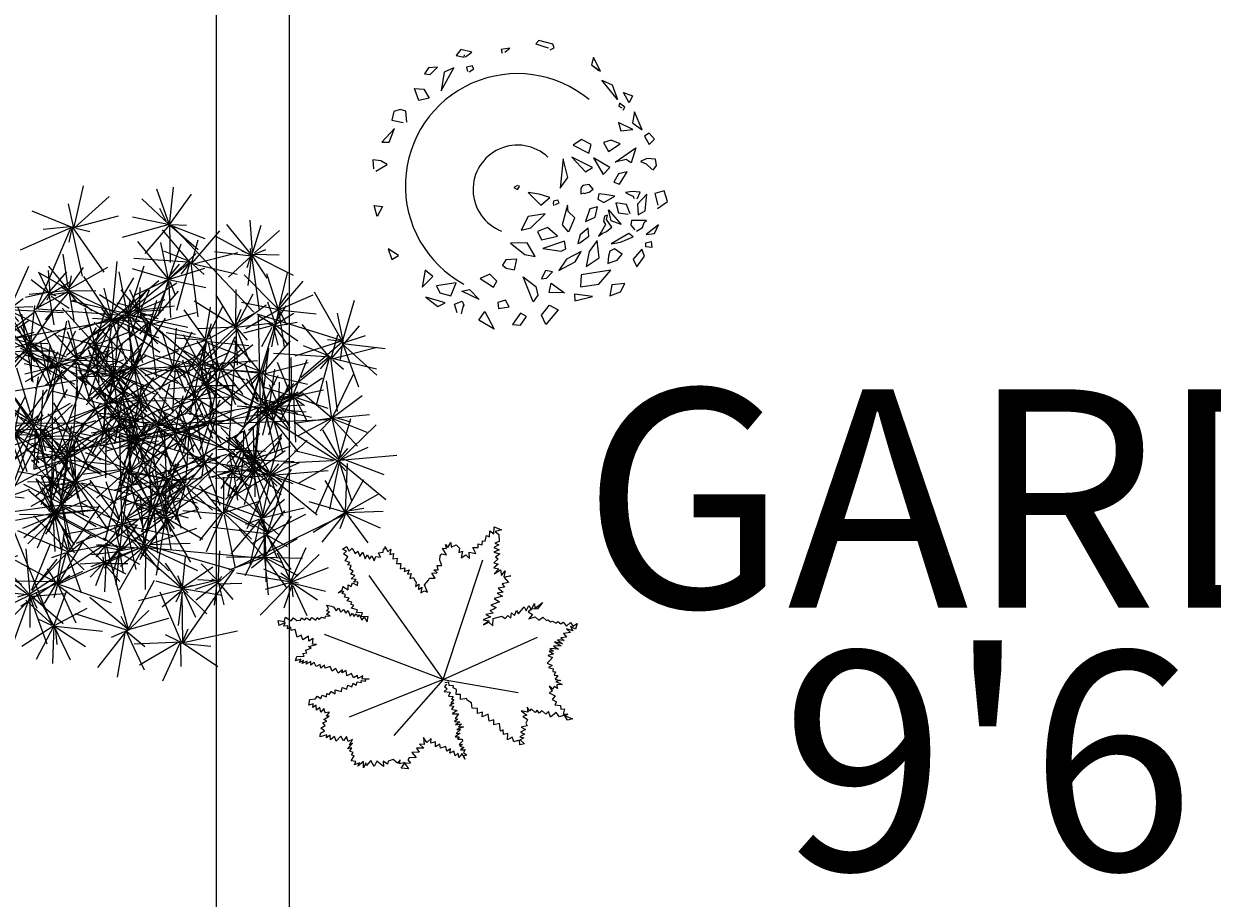
# Model space of a CAD drawing. Units: inches. Extents: x 8049 to 8459, y 820 to 1350.
# Tile 15 of 25: x 8132 to 8165, y 906 to 930. Entities that reach past the tile are written whole.
import ezdxf

# ---------------------------------------------------------------- set-up
doc = ezdxf.new("R2010")
doc.units = ezdxf.units.IN
doc.header["$MEASUREMENT"] = 0
for name, color, linetype, lineweight in [('A-ANNO-DIMS', 2, 'Continuous', 18), ('A-AREA-IDEN', 7, 'Continuous', 25), ('zelen', 69, 'Continuous', 13)]:
    doc.layers.add(name, color=color, linetype=linetype, lineweight=lineweight)
doc.styles.get("Standard").update_dxf_attribs({"font": 'arial.ttf'})
doc.dimstyles.get("Standard").update_dxf_attribs({"dimtxt": 0.18, "dimasz": 0.18, "dimexe": 0.18, "dimexo": 0.0625, "dimgap": 0.09, "dimtad": 0, "dimtih": 1, "dimtoh": 1, "dimdec": 4, "dimzin": 0, "dimdsep": 46, "dimtxsty": 'Standard', "dimcen": 0.09, "dimadec": 0, "dimazin": 0, "dimtfac": 1, "dimtdec": 4, "dimtofl": 0, "dimtmove": 0, "dimatfit": 3, "dimfxl": 1, "dimtolj": 1, "dimtzin": 0, "dimarcsym": 0})

# ---------------------------------------------------------------- blocks, each defined once
blk = doc.blocks.new('z_85')
for p, q in [((140.4, 459.9), (144.1, 478.3)), ((144.1, 478.3), (154.8, 474.2)), ((154.8, 474.2), (155.6, 493.8)), ((155.6, 493.8), (168.5, 483.9)), ((168.5, 483.9), (169.7, 507.5)), ((169.7, 507.5), (194.7, 497.5)), ((194.7, 497.5), (173, 491.4)), ((173, 491.4), (185.2, 481.2)), ((185.2, 481.2), (186.9, 458.5)), ((-334.5, 433), (-320.5, 441.8)), ((-320.5, 441.8), (-312.2, 426.3)), ((-312.2, 426.3), (-302, 436.4)), ((-302, 436.4), (-292.5, 418.9)), ((-192.6, 433.8), (-192.5, 442.2)), ((-192.5, 442.2), (-183.3, 424.5)), ((-2.1, 435.8), (11.7, 434.9)), ((11.4, 414.5), (-2.1, 435.8)), ((8.4, 449), (15.4, 438)), ((11.7, 434.9), (8.4, 449)), ((15.4, 438), (25.6, 455.6)), ((25.6, 455.6), (26.4, 439.7)), ((26.4, 439.7), (44.1, 447.4)), ((44.1, 447.4), (54.4, 436.3)), ((54.4, 436.3), (52.3, 421.7)), ((98.5, 438.8), (116.6, 438)), ((108.9, 418.4), (98.5, 438.8)), ((116.1, 450.2), (130, 447.6)), ((116.6, 438), (116.1, 450.2)), ((130, 447.6), (130.9, 460.7)), ((130.9, 460.7), (140.4, 459.9)), ((185.1, 447.3), (169, 438)), ((169, 438), (186.4, 430.3)), ((186.9, 458.5), (172.1, 453.2)), ((172.1, 453.2), (185.1, 447.3)), ((-320.3, 426.3), (-334.5, 433)), ((-331, 417), (-320.3, 426.3)), ((-316.9, 407.2), (-331, 417)), ((-325.3, 394.5), (-316.9, 407.2)), ((-292.5, 418.9), (-282.7, 426.1)), ((-282.7, 426.1), (-277, 408.1)), ((-277, 408.1), (-266.3, 423.5)), ((-266.3, 423.5), (-258.7, 400.7)), ((-258.7, 400.7), (-250.8, 414.2)), ((-250.8, 414.2), (-244.9, 399.8)), ((-244.9, 399.8), (-237.2, 410.8)), ((-237.2, 410.8), (-228.5, 393.9)), ((-228.5, 393.9), (-223.5, 408.6)), ((-223.5, 408.6), (-207.8, 406.4)), ((-214.2, 421.3), (-198.5, 423)), ((-207.8, 406.4), (-214.2, 421.3)), ((-198.5, 423), (-198.2, 434.1)), ((-198.2, 434.1), (-192.6, 433.8)), ((-183.3, 424.5), (-173.3, 433.2)), ((-173.3, 433.2), (-176.4, 415.5)), ((-176.4, 415.5), (-165.1, 418.9)), ((-165.1, 418.9), (-166.4, 400.3)), ((-166.4, 400.3), (-152.4, 402.8)), ((-152.4, 402.8), (-154.8, 385.2)), ((-10.8, 396), (-9.6, 410.9)), ((-4.1, 379.1), (-10.8, 396)), ((-9.6, 410.9), (-3.8, 416.9)), ((-3.8, 416.9), (11.4, 414.5)), ((0, 0), (132.7, 397)), ((52.3, 421.7), (64.6, 426)), ((64.6, 426), (59.8, 403.9)), ((59.8, 403.9), (75.6, 414.2)), ((75.6, 414.2), (88.3, 401.4)), ((86.4, 422.5), (108.9, 418.4)), ((88.3, 401.4), (86.4, 422.5)), ((186.4, 430.3), (169.1, 422.7)), ((169.1, 422.7), (188.1, 417.5)), ((183.6, 400.7), (169.1, 387.1)), ((188.1, 417.5), (174.5, 406.5)), ((174.5, 406.5), (183.6, 400.7)), ((-309.5, 388.7), (-325.3, 394.5)), ((-317.2, 380.4), (-309.5, 388.7)), ((-305.1, 378.2), (-317.2, 380.4)), ((-309.5, 366.8), (-305.1, 378.2)), ((-299.2, 360.3), (-309.5, 366.8)), ((-305.9, 349.8), (-299.2, 360.3)), ((-154.8, 385.2), (-139.8, 385.6)), ((-139.8, 385.6), (-142, 367.5)), ((-142, 367.5), (-126.8, 370.7)), ((-126.8, 370.7), (-129.7, 358.9)), ((-129.7, 358.9), (-112.6, 364.1)), ((-112.6, 364.1), (-118.7, 349.7)), ((-31.2, 364.3), (-16.4, 364.7)), ((-19.6, 354.2), (-31.2, 364.3)), ((-19.9, 378.2), (-4.1, 379.1)), ((-16.4, 364.7), (-19.9, 378.2)), ((182.7, 383.5), (168.5, 371)), ((168.5, 371), (185.5, 367.5)), ((169.1, 387.1), (182.7, 383.5)), ((185.5, 367.5), (169.7, 351.3)), ((169.7, 351.3), (191.1, 364.1)), ((191.1, 364.1), (194, 345.3)), ((194, 345.3), (206.3, 360.8)), ((206.3, 360.8), (201.7, 341.2)), ((-292.6, 345.9), (-305.9, 349.8)), ((-305.3, 333.9), (-292.6, 345.9)), ((-288.9, 332.3), (-305.3, 333.9)), ((-305, 309.4), (-300.9, 321)), ((-300.9, 321), (-284.3, 312.7)), ((-296.8, 323.1), (-288.9, 332.3)), ((-283.1, 324), (-296.8, 323.1)), ((-284.3, 312.7), (-283.1, 324)), ((0, 0), (-245.8, 345.3)), ((-118.7, 349.7), (-106.5, 351.7)), ((-106.5, 351.7), (-110.4, 335.8)), ((-110.4, 335.8), (-98.6, 339.2)), ((-98.6, 339.2), (-92.9, 326.8)), ((-92.9, 326.8), (-89.6, 322.3)), ((-89.6, 322.3), (-91.1, 309)), ((-91.1, 309), (-80.4, 316.3)), ((-80.4, 316.3), (-81.2, 298.5)), ((-61.6, 314), (-48.8, 329.6)), ((-48.8, 329.6), (-45, 336.2)), ((-45, 336.2), (-26.1, 337)), ((-37.5, 352.7), (-19.6, 354.2)), ((-26.1, 337), (-37.5, 352.7)), ((217.5, 321.8), (196.8, 317.3)), ((196.8, 317.3), (204.7, 306.3)), ((201.7, 341.2), (224.8, 344.2)), ((224.8, 344.2), (203.2, 339.2)), ((203.2, 339.2), (217.5, 321.8)), ((-348.8, 287.5), (-334.3, 298.5)), ((-329.7, 291.9), (-348.8, 287.5)), ((-335.7, 285.2), (-329.7, 291.9)), ((-323.9, 282.5), (-335.7, 285.2)), ((-334.3, 298.5), (-333.4, 308.7)), ((-333.4, 308.7), (-315.2, 298.3)), ((-327.7, 273.4), (-323.9, 282.5)), ((-315.2, 298.3), (-314.9, 314.1)), ((-314.9, 314.1), (-305, 309.4)), ((-81.2, 298.5), (-70.2, 306.6)), ((-70.2, 306.6), (-73.6, 287.8)), ((-73.6, 287.8), (-62, 294.6)), ((-62, 294.6), (-51.7, 290.2)), ((-51.7, 290.2), (-61.6, 314)), ((199.8, 290.5), (179.5, 286.4)), ((179.5, 286.4), (198, 276.2)), ((204.7, 306.3), (183.1, 303.2)), ((183.1, 303.2), (199.8, 290.5)), ((-386.6, 246.8), (-370.9, 243.8)), ((-380.3, 234.1), (-386.6, 246.8)), ((-370.9, 243.8), (-362.5, 240.1)), ((-362.5, 240.1), (-355.4, 227.7)), ((-355.4, 227.7), (-347.7, 237.1)), ((-347.7, 237.1), (-340.1, 223.9)), ((-312.5, 269.8), (-327.7, 273.4)), ((-318.1, 260.9), (-312.5, 269.8)), ((-303.5, 257.1), (-318.1, 260.9)), ((-306.9, 250.2), (-303.5, 257.1)), ((-296.5, 245.4), (-306.9, 250.2)), ((-304.8, 236.9), (-296.5, 245.4)), ((-284, 230.8), (-304.8, 236.9)), ((187.9, 258.2), (158.6, 247.3)), ((158.6, 247.3), (176.5, 239.3)), ((176.5, 239.3), (169.1, 234)), ((198, 276.2), (169.3, 269.4)), ((169.3, 269.4), (187.9, 258.2)), ((251.2, 218.3), (269.1, 241.8)), ((269.1, 241.8), (276.1, 228.2)), ((276.1, 228.2), (284.6, 245.4)), ((284.6, 245.4), (292.5, 230.8)), ((292.5, 230.8), (304.2, 252.6)), ((304.2, 252.6), (305.4, 235.8)), ((305.4, 235.8), (330.6, 255.3)), ((330.6, 255.3), (314, 234.4)), ((-527.9, 192.6), (-523, 206.4)), ((-523, 206.4), (-504.7, 194.2)), ((-504.7, 194.2), (-496.5, 204.8)), ((-496.5, 204.8), (-486, 196.2)), ((-473.8, 197.3), (-470.6, 205)), ((-470.6, 205), (-459, 197.9)), ((-459, 197.9), (-453.2, 204.7)), ((-453.2, 204.7), (-441.7, 197.3)), ((-441.7, 197.3), (-436, 206.1)), ((-436, 206.1), (-423, 196.7)), ((-423, 196.7), (-417.9, 205.5)), ((-417.9, 205.5), (-411.3, 200.8)), ((-411.3, 200.8), (-403.9, 207.3)), ((-403.9, 207.3), (-392, 203.9)), ((-392, 203.9), (-391, 210.5)), ((-391, 210.5), (-375.1, 210.9)), ((-387.5, 216.4), (-377.3, 224.9)), ((-375.1, 210.9), (-387.5, 216.4)), ((-387.2, 228.2), (-380.3, 234.1)), ((-377.3, 224.9), (-387.2, 228.2)), ((-340.1, 223.9), (-331.2, 232.1)), ((-331.2, 232.1), (-323, 219.9)), ((-323, 219.9), (-314.9, 229.4)), ((-314.9, 229.4), (-308.7, 210.5)), ((-308.7, 210.5), (-301.4, 220.5)), ((-301.4, 220.5), (-296.2, 209.5)), ((-296.2, 209.5), (-288.7, 218.5)), ((-288.7, 218.5), (-282.8, 208)), ((-287.5, 222.7), (-284, 230.8)), ((-267.9, 221.3), (-287.5, 222.7)), ((-282.8, 208), (-278.3, 215.3)), ((-278.3, 215.3), (-269.6, 197)), ((-272.7, 208.1), (-267.9, 221.3)), ((-249.1, 208.6), (-272.7, 208.1)), ((-269.6, 197), (-261.6, 206.7)), ((-261.6, 206.7), (-252.6, 191.1)), ((-252.6, 191.1), (-249.1, 208.6)), ((157.5, 207.7), (133, 198.3)), ((133, 198.3), (152.7, 194.8)), ((166.6, 220), (142.5, 215.8)), ((142.5, 215.8), (157.5, 207.7)), ((169.1, 234), (156.5, 228.6)), ((156.5, 228.6), (166.6, 220)), ((165.5, 178.4), (166.1, 202.2)), ((166.1, 202.2), (195.8, 210)), ((195.8, 210), (206.3, 202.3)), ((206.3, 202.3), (214.9, 212.7)), ((214.9, 212.7), (225, 203.7)), ((225, 203.7), (227.4, 221.4)), ((227.4, 221.4), (237.6, 211.9)), ((237.6, 211.9), (244, 229.6)), ((244, 229.6), (251.2, 218.3)), ((291.9, 231.3), (282.8, 224.3)), ((282.8, 224.3), (297.7, 215.3)), ((297.7, 215.3), (285.2, 201.4)), ((285.2, 201.4), (305.7, 207.8)), ((294, 233.8), (291.9, 231.3)), ((314, 234.4), (294, 233.8)), ((305.7, 207.8), (318.4, 196.7)), ((318.4, 196.7), (331.5, 207.2)), ((331.5, 207.2), (343.4, 195.3)), ((343.4, 195.3), (349.2, 197.8)), ((349.2, 197.8), (357.1, 191.7)), ((-547.4, 195.4), (-527.9, 192.6)), ((-544.7, 179.5), (-547.4, 195.4)), ((-524.7, 189.5), (-544.7, 179.5)), ((-528.5, 176.6), (-524.7, 189.5)), ((-515.5, 177.6), (-528.5, 176.6)), ((-516.7, 167.9), (-515.5, 177.6)), ((-506.3, 173.2), (-516.7, 167.9)), ((-504.7, 162.4), (-506.3, 173.2)), ((-491.4, 165.7), (-504.7, 162.4)), ((-484.9, 140.6), (-491.4, 165.7)), ((-486, 196.2), (-473.8, 197.3)), ((152.7, 194.8), (134.2, 181.8)), ((134.2, 181.8), (152.3, 190.3)), ((152.3, 190.3), (165.5, 178.4)), ((357.1, 191.7), (363.4, 194)), ((363.4, 194), (375.4, 187.3)), ((375.4, 187.3), (381.6, 192.9)), ((381.6, 192.9), (391.6, 185.1)), ((391.6, 185.1), (399.5, 189.8)), ((399.5, 189.8), (410.7, 177.1)), ((410.7, 177.1), (423.8, 189)), ((410.7, 167.7), (422.9, 156)), ((431.6, 161.5), (410.7, 167.7)), ((423.8, 189), (430.9, 177.3)), ((423.8, 175.6), (431.6, 161.5)), ((440.2, 166.6), (423.8, 175.6)), ((430.9, 177.3), (445.2, 185.4)), ((445.2, 185.4), (440.2, 166.6)), ((-472, 147), (-484.9, 140.6)), ((-466.4, 131.1), (-472, 147)), ((-447.4, 143.9), (-466.4, 131.1)), ((-446.4, 127.5), (-447.4, 143.9)), ((-431.2, 136.1), (-446.4, 127.5)), ((-433.6, 116.8), (-432.5, 124.7)), ((-432.5, 124.7), (-431.2, 136.1)), ((0, 0), (-394.4, 149.4)), ((0, 0), (313.9, 140.8)), ((370, 124.5), (392.9, 111.3)), ((397.4, 117.9), (370, 124.5)), ((380.7, 131.9), (397.4, 117.9)), ((402.3, 129), (380.7, 131.9)), ((410.7, 140.5), (391.1, 138)), ((391.1, 138), (402.3, 129)), ((422.9, 156), (399.8, 152.7)), ((399.8, 152.7), (410.7, 140.5)), ((-466.3, 86.6), (-452.6, 88.2)), ((-461.1, 77.2), (-466.3, 86.6)), ((-456.8, 97.3), (-437.9, 103.7)), ((-452.6, 88.2), (-456.8, 97.3)), ((-447.3, 109), (-420.9, 115.7)), ((-437.9, 103.7), (-447.3, 109)), ((-420.9, 115.7), (-433.6, 116.8)), ((367.5, 85.5), (348.2, 79.7)), ((348.2, 79.7), (364, 72.5)), ((367.3, 93.6), (352.7, 93.5)), ((352.7, 93.5), (367.5, 85.5)), ((354.4, 102.3), (367.3, 93.6)), ((384, 100.5), (354.4, 102.3)), ((392.9, 111.3), (367, 110.4)), ((367, 110.4), (384, 100.5)), ((-490.1, 61.5), (-485.7, 76.6)), ((-472.7, 67.7), (-490.1, 61.5)), ((-485.7, 76.6), (-461.1, 77.2)), ((-477.3, 56.2), (-472.7, 67.7)), ((-464.1, 63.3), (-477.3, 56.2)), ((-468.4, 52.6), (-464.1, 63.3)), ((-452, 61.1), (-468.4, 52.6)), ((-455.1, 51.2), (-452, 61.1)), ((-439, 59.8), (-455.1, 51.2)), ((-439.5, 47.5), (-439, 59.8)), ((-428.5, 56.1), (-439.5, 47.5)), ((-421.5, 42.4), (-428.5, 56.1)), ((-408.4, 49.5), (-421.5, 42.4)), ((-406.6, 37.3), (-408.4, 49.5)), ((-393.5, 46.8), (-406.6, 37.3)), ((-392.2, 37), (-393.5, 46.8)), ((-375.3, 43.4), (-392.2, 37)), ((-368.7, 27.4), (-375.3, 43.4)), ((355.3, 62.8), (346.4, 53.6)), ((346.4, 53.6), (362.3, 46.4)), ((362.3, 46.4), (350.4, 40.1)), ((350.4, 40.1), (365.4, 35.2)), ((364, 72.5), (355.3, 62.8)), ((-356.3, 36.3), (-368.7, 27.4)), ((-348.5, 20.8), (-356.3, 36.3)), ((-333.9, 32.3), (-348.5, 20.8)), ((-335.5, 21.5), (-333.9, 32.3)), ((-322.4, 29.1), (-335.5, 21.5)), ((-319.9, 12.2), (-322.4, 29.1)), ((-303.8, 20), (-319.9, 12.2)), ((0, 0), (-312.2, -125)), ((-297.7, 5.3), (-303.8, 20)), ((-284.2, 12.8), (-297.7, 5.3)), ((-282.8, 2.5), (-284.2, 12.8)), ((-266.1, 11.6), (-282.8, 2.5)), ((-268.5, 0.9), (-266.1, 11.6)), ((-245.2, 1.9), (-268.5, 0.9)), ((-258.6, 1.3), (-245.2, 1.9)), ((-256.6, -5.5), (-258.6, 1.3)), ((0, 0), (-163.1, -186)), ((0, 0), (249.7, -43.2)), ((365.4, 35.2), (364.6, 26)), ((364.6, 26), (373.9, 25.2)), ((373.9, 25.2), (368.8, 14.6)), ((368.8, 14.6), (381.5, 13.5)), ((381.5, 13.5), (372.3, 1.1)), ((372.3, 1.1), (390.8, -3.1)), ((-358.6, -35.2), (-337, -39.8)), ((-358.3, -47.6), (-358.6, -35.2)), ((-337, -39.8), (-335.4, -26.5)), ((-335.4, -26.5), (-320, -32.7)), ((-320, -32.7), (-316.6, -19.6)), ((-316.6, -19.6), (-303.5, -24.4)), ((-303.5, -24.4), (-299.1, -12.1)), ((-299.1, -12.1), (-288.4, -18.9)), ((-288.4, -18.9), (-284.9, -7.8)), ((-284.9, -7.8), (-270.6, -10.5)), ((-272, -3.8), (-256.6, -5.5)), ((-270.6, -10.5), (-272, -3.8)), ((14.2, -31.5), (3.8, -40.4)), ((11, -15.5), (4.4, -23.3)), ((4.4, -23.3), (14.2, -31.5)), ((19.4, -9.1), (6, -11.1)), ((20.6, -19.7), (19.4, -9.1)), ((34.5, -21), (20.6, -19.7)), ((33.9, -27.7), (34.5, -21)), ((44.7, -33.5), (33.9, -27.7)), ((43.2, -50.4), (44.7, -33.5)), ((352.1, -22.6), (362.5, -39.2)), ((365.2, -32.7), (352.1, -22.6)), ((362.5, -39.2), (352.9, -44.5)), ((368.7, -23.2), (365.2, -32.7)), ((380.7, -30.1), (368.7, -23.2)), ((390.8, -3.1), (374.2, -7.2)), ((374.2, -7.2), (396.2, -16.9)), ((378.3, -17.7), (377.9, -21.9)), ((377.9, -21.9), (380.7, -30.1)), ((396.2, -16.9), (378.3, -17.7)), ((-445.6, -85.2), (-442.8, -66.9)), ((-442.8, -66.9), (-423.6, -64.7)), ((-423.6, -64.7), (-418.1, -55.3)), ((-418.1, -55.3), (-406.6, -63.9)), ((-406.6, -63.9), (-402.1, -52.8)), ((-402.1, -52.8), (-387.5, -58.3)), ((-387.5, -58.3), (-386, -47.3)), ((-386, -47.3), (-378.3, -50.6)), ((-378.3, -50.6), (-371.8, -40.4)), ((-371.8, -40.4), (-358.3, -47.6)), ((3.8, -40.4), (23.3, -42)), ((23.3, -42), (17.8, -55.3)), ((17.8, -55.3), (33.3, -57.2)), ((35.8, -67.3), (26.2, -78.5)), ((26.2, -78.5), (35.4, -79.2)), ((33.3, -57.2), (27.6, -66.1)), ((27.6, -66.1), (35.8, -67.3)), ((57.8, -49.8), (43.2, -50.4)), ((57.8, -66.7), (57.8, -49.8)), ((79.4, -63.3), (57.8, -66.7)), ((80.6, -68.6), (79.4, -63.3)), ((95, -77.7), (80.6, -68.6)), ((96.5, -95.7), (95, -77.7)), ((352.9, -44.5), (372.4, -54.8)), ((372.4, -54.8), (362.2, -67.3)), ((362.2, -67.3), (377.4, -74.9)), ((377.4, -74.9), (371.4, -84.3)), ((-431.8, -81.7), (-445.6, -85.2)), ((-433, -93.3), (-431.8, -81.7)), ((-421.5, -86.1), (-433, -93.3)), ((-420.3, -102.3), (-421.5, -86.1)), ((-408.9, -93.6), (-420.3, -102.3)), ((-406.5, -108.7), (-408.9, -93.6)), ((-396.2, -96.8), (-406.5, -108.7)), ((-391.4, -111), (-396.2, -96.8)), ((-377.3, -108.5), (-391.4, -111)), ((-387.6, -122.5), (-377.3, -108.5)), ((35.4, -79.2), (20.9, -86.9)), ((20.9, -86.9), (36.1, -88.5)), ((36.1, -88.5), (28.2, -99.3)), ((28.2, -99.3), (46.8, -102.9)), ((31.9, -112.9), (31.3, -114)), ((31.3, -114), (51.4, -114.8)), ((46.8, -102.9), (31.9, -112.9)), ((51.4, -114.8), (39.8, -130.3)), ((114.9, -96.9), (96.5, -95.7)), ((113.9, -113.2), (114.9, -96.9)), ((131.6, -109.3), (113.9, -113.2)), ((129.5, -124.2), (131.6, -109.3)), ((150, -116), (129.5, -124.2)), ((153.5, -138.6), (150, -116)), ((259.9, -104.5), (278.9, -118.5)), ((281.6, -108.4), (259.9, -104.5)), ((279.1, -92.7), (281.6, -108.4)), ((288.4, -105.6), (279.1, -92.7)), ((292.3, -97.7), (288.4, -105.6)), ((306.3, -109.8), (292.3, -97.7)), ((312.3, -101.9), (306.3, -109.8)), ((319.1, -112.6), (312.3, -101.9)), ((329.4, -104.1), (319.1, -112.6)), ((341.7, -115.9), (329.4, -104.1)), ((350.6, -106.3), (341.7, -115.9)), ((357.5, -125.6), (350.6, -106.3)), ((375.9, -109.5), (357.5, -125.6)), ((371.4, -84.3), (390.2, -87.1)), ((386.6, -123.9), (375.9, -109.5)), ((390.2, -87.1), (391, -98.7)), ((391, -98.7), (403.6, -97.7)), ((403.6, -97.7), (399.4, -115.7)), ((399.4, -115.7), (414.2, -115.6)), ((414.2, -115.6), (406.2, -120.7)), ((-405.7, -161.9), (-391.7, -153.5)), ((-399.4, -144.9), (-386, -138.6)), ((-391.7, -153.5), (-399.4, -144.9)), ((-396.7, -133.3), (-378.8, -121.8)), ((-386, -138.6), (-396.7, -133.3)), ((-378.8, -121.8), (-387.6, -122.5)), ((49.4, -132), (38, -139.7)), ((38, -139.7), (55.7, -140.9)), ((39.8, -130.3), (49.4, -132)), ((55.7, -140.9), (40.8, -150.5)), ((40.8, -150.5), (61.7, -147.7)), ((67.9, -157.4), (45.5, -166.6)), ((61.7, -147.7), (51.2, -158.2)), ((51.2, -158.2), (67.9, -157.4)), ((168.2, -134.7), (153.5, -138.6)), ((168.7, -151.1), (168.2, -134.7)), ((187.2, -147), (168.7, -151.1)), ((190.4, -171.9), (187.2, -147)), ((279.5, -153.9), (259.5, -159.1)), ((278.9, -118.5), (264.8, -122.8)), ((264.8, -122.8), (279.4, -131.9)), ((280.4, -134.4), (275.3, -145.6)), ((275.3, -145.6), (279.5, -153.9)), ((279.4, -131.9), (280.4, -134.4)), ((403.8, -118.5), (386.6, -123.9)), ((413.1, -135.8), (403.8, -118.5)), ((406.2, -120.7), (430, -130.9)), ((430, -130.9), (413.1, -135.8)), ((-408.7, -191.2), (-407.1, -178.7)), ((-386.3, -183.7), (-408.7, -191.2)), ((-407.1, -178.7), (-394, -170.7)), ((-394, -170.7), (-405.7, -161.9)), ((-386.9, -194.2), (-386.3, -183.7)), ((-375, -185.4), (-386.9, -194.2)), ((-374.4, -200.4), (-375, -185.4)), ((-361, -190), (-374.4, -200.4)), ((-355.6, -205.5), (-361, -190)), ((-340.1, -188.9), (-355.6, -205.5)), ((-331, -204.2), (-340.1, -188.9)), ((-320.5, -190.1), (-331, -204.2)), ((-315.8, -206.4), (-320.5, -190.1)), ((-64.5, -193.4), (-63.1, -216.4)), ((-54.1, -209.7), (-64.5, -193.4)), ((-39.9, -196.5), (-54.1, -209.7)), ((-40.4, -212.5), (-39.9, -196.5)), ((57.1, -178.7), (40.5, -191.1)), ((40.5, -191.1), (53.9, -190.4)), ((57.7, -166.9), (43.5, -179.6)), ((43.5, -179.6), (57.1, -178.7)), ((45.5, -166.6), (57.7, -166.9)), ((53.9, -190.4), (47.9, -199)), ((199.5, -167.6), (190.4, -171.9)), ((201.2, -183.5), (199.5, -167.6)), ((215.4, -180.2), (201.2, -183.5)), ((214.3, -200.6), (215.4, -180.2)), ((229.7, -192.5), (214.3, -200.6)), ((235.5, -207.5), (229.7, -192.5)), ((270.6, -182.1), (255.6, -190.7)), ((255.6, -190.7), (268.7, -194.5)), ((268.7, -194.5), (256, -201.4)), ((273.9, -166.2), (257.2, -175.1)), ((257.2, -175.1), (270.6, -182.1)), ((259.5, -159.1), (273.9, -166.2)), ((-316.4, -230.7), (-301.2, -212.5)), ((-303, -227.7), (-316.4, -230.7)), ((-300.9, -199.4), (-315.8, -206.4)), ((-311, -217.5), (-300.9, -199.4)), ((-301.2, -212.5), (-311, -217.5)), ((-309.9, -238.3), (-303, -227.7)), ((-63.4, -228.2), (-87.9, -229.1)), ((-87.9, -229.1), (-79.8, -242)), ((-78.5, -215.2), (-63.4, -228.2)), ((-63.1, -216.4), (-78.5, -215.2)), ((-25.3, -207.7), (-40.4, -212.5)), ((-25.3, -223.8), (-25.3, -207.7)), ((-10.7, -215.8), (-25.3, -223.8)), ((-8.3, -228.6), (-10.7, -215.8)), ((8.9, -223.5), (-8.3, -228.6)), ((12.7, -238.7), (8.9, -223.5)), ((24.7, -230.5), (12.7, -238.7)), ((23, -244.8), (24.7, -230.5)), ((47.9, -199), (63.4, -198.7)), ((65.1, -205.6), (53.6, -216.1)), ((53.6, -216.1), (64.9, -216.9)), ((64.9, -216.9), (56, -222.4)), ((56, -222.4), (69.4, -226.9)), ((69.4, -226.9), (58.1, -234.3)), ((58.1, -234.3), (70.9, -234.4)), ((63.4, -198.7), (65.1, -205.6)), ((73.9, -233.5), (67.9, -243.4)), ((70.9, -234.4), (73.9, -233.5)), ((253.5, -202), (235.5, -207.5)), ((255.4, -217.1), (253.5, -202)), ((270.6, -214.1), (255.4, -217.1)), ((256, -201.4), (270.6, -214.1)), ((-298.3, -242.6), (-309.9, -238.3)), ((-305.3, -270.9), (-295, -254.3)), ((-290.1, -273.1), (-305.3, -270.9)), ((-304.7, -251.3), (-298.3, -242.6)), ((-295, -254.3), (-304.7, -251.3)), ((-294.6, -284.2), (-290.1, -273.1)), ((-264.9, -273), (-283.1, -288.1)), ((-264.3, -294.3), (-264.9, -273)), ((-239.6, -270.1), (-254.5, -286.6)), ((-228.6, -289.1), (-239.6, -270.1)), ((-220, -272), (-228.6, -289.1)), ((-197.9, -289.9), (-220, -272)), ((-199.2, -272), (-197.9, -289.9)), ((-184.2, -282), (-199.2, -272)), ((-182.4, -271.4), (-184.2, -282)), ((-166.3, -266.5), (-182.4, -271.4)), ((-151.2, -278.6), (-166.3, -266.5)), ((-142.3, -267.5), (-151.2, -278.6)), ((-144.6, -280.3), (-142.3, -267.5)), ((-126.2, -276.2), (-144.6, -280.3)), ((-138.9, -294.9), (-126.2, -276.2)), ((-113.1, -261.1), (-117.3, -267.5)), ((-117.3, -267.5), (-107.8, -278)), ((-88.9, -260), (-113.1, -261.1)), ((-79.8, -242), (-103.3, -242.6)), ((-103.3, -242.6), (-88.9, -260)), ((35.5, -238.8), (23, -244.8)), ((40.7, -254.5), (35.5, -238.8)), ((49.8, -244.9), (40.7, -254.5)), ((52.7, -259.2), (49.8, -244.9)), ((63.6, -245.9), (52.7, -259.2)), ((72.4, -265), (63.6, -245.9)), ((67.9, -243.4), (79.4, -252.4)), ((79.4, -252.4), (68.2, -253.9)), ((68.2, -253.9), (72.4, -265)), ((-277.1, -277.7), (-294.6, -284.2)), ((-283.1, -288.1), (-277.1, -277.7)), ((-256.6, -277.5), (-264.3, -294.3)), ((-254.5, -286.6), (-256.6, -277.5)), ((-114.3, -296.8), (-138.9, -294.9)), ((-107.8, -278), (-127.3, -279.2)), ((-127.3, -279.2), (-114.3, -296.8))]:
    blk.add_line(p, q)
blk = doc.blocks.new('z_66')
for p, q in [((83.2, 488.9), (72.7, 477.7)), ((72.7, 477.7), (96.4, 469.7)), ((129.8, 476.2), (83.2, 488.9)), ((134, 464.6), (129.8, 476.2)), ((-176.4, 458.5), (-191.7, 438.6)), ((-191.7, 438.6), (-165.6, 433.5)), ((-139.2, 449.4), (-176.4, 458.5)), ((-165.6, 433.5), (-163.6, 441.1)), ((-161.1, 434.6), (-139.2, 449.4)), ((-13.6, 463.6), (-42.5, 459.2)), ((-42.5, 459.2), (-39.3, 446.9)), ((-30.3, 449.4), (-13.6, 463.6)), ((96.4, 469.7), (114.5, 463.9)), ((114.5, 463.9), (114.5, 463.9)), ((120.4, 457.8), (134, 464.6)), ((-283.6, 397.7), (-297.2, 378.2)), ((-254, 399.9), (-283.6, 397.7)), ((-272.8, 380.7), (-254, 399.9)), ((-241.9, 321.7), (-199.1, 397.3)), ((-199.1, 397.3), (-231.4, 383.6)), ((-165.6, 433.5), (-165.6, 433.5)), ((-138.9, 404.9), (-156.9, 400.2)), ((-156.9, 400.2), (-153.8, 385.4)), ((-133.3, 394.8), (-138.9, 404.9)), ((265.2, 432.1), (258.2, 407.5)), ((258.2, 407.5), (287.4, 387.2)), ((258.2, 407.5), (281.9, 388.6)), ((287.4, 387.2), (265.2, 432.1)), ((-297.2, 378.2), (-277.7, 376)), ((-277.7, 376), (-272.8, 380.7)), ((-231.4, 383.6), (-241.9, 321.7)), ((-148.6, 384.7), (-133.3, 394.8)), ((281.9, 388.6), (281.9, 388.6)), ((344.2, 293.1), (292, 357.2)), ((292, 357.2), (326.8, 341.2)), ((-330.3, 328.9), (-298.6, 327.1)), ((-316, 288.8), (-330.3, 328.9)), ((-298.6, 327.1), (-280.8, 297.1)), ((326.8, 341.2), (344.2, 293.1)), ((383.1, 281.9), (364.4, 316.3)), ((364.4, 316.3), (394.6, 305.1)), ((-280.8, 297.1), (-316, 288.8)), ((350.8, 280.8), (348.7, 270.3)), ((369.2, 266.7), (350.8, 280.8)), ((394.6, 305.1), (383.1, 281.9)), ((-399.2, 252.6), (-405.8, 224)), ((-377.9, 259.1), (-399.2, 252.6)), ((-358.4, 254), (-377.9, 259.1)), ((-356, 217.5), (-358.4, 254)), ((348.7, 270.3), (358.8, 264.5)), ((358.8, 264.5), (358.8, 264.5)), ((363.3, 256.6), (369.2, 266.7)), ((400.9, 251.9), (393.9, 214.6)), ((426.6, 192.2), (400.9, 251.9)), ((-405.8, 224), (-368.2, 216.4)), ((-368.2, 216.4), (-368.2, 216.4)), ((348, 215.7), (356, 188.9)), ((395.3, 193.2), (348, 215.7)), ((393.9, 214.6), (426.6, 192.2)), ((-396.4, 196.1), (-438.1, 150.2)), ((-414.8, 150.9), (-396.4, 196.1)), ((225.2, 159.9), (197, 140.8)), ((256.8, 142.6), (225.2, 159.9)), ((356, 188.9), (395.3, 193.2)), ((450, 180.6), (434.3, 171.2)), ((434.3, 171.2), (449.6, 142.6)), ((449.6, 142.6), (467.7, 160.3)), ((467.7, 160.3), (450, 180.6)), ((-438.1, 150.2), (-414.8, 150.9)), ((197, 140.8), (249.5, 113.6)), ((249.5, 113.6), (256.8, 142.6)), ((323.6, 157.8), (297.5, 149.8)), ((297.5, 149.8), (314.6, 119.4)), ((314.6, 119.4), (352.9, 145.5)), ((352.9, 145.5), (323.6, 157.8)), ((336.9, 84.3), (405.8, 131.7)), ((405.8, 131.7), (389.8, 82.1)), ((-468.4, 91.6), (-466.3, 62.6)), ((-441.6, 89), (-468.4, 91.6)), ((-421.1, 76), (-441.6, 89)), ((164.3, 94.8), (154.2, -2.2)), ((178.9, 33.3), (164.3, 94.8)), ((193.1, 101.3), (238, 52.1)), ((261.7, 66.6), (193.1, 101.3)), ((265.2, 98.8), (297.2, 42.7)), ((318.8, 66.2), (265.2, 98.8)), ((372.7, 93), (336.9, 84.3)), ((389.8, 82.1), (372.7, 93)), ((441.6, 95.9), (420.7, 86.5)), ((420.7, 86.5), (440.2, 78.5)), ((470.5, 93.7), (441.6, 95.9)), ((474, 73.5), (470.5, 93.7)), ((-466.3, 62.6), (-466.3, 62.6)), ((-458.3, 53.9), (-421.1, 76)), ((238, 52.1), (261.7, 66.6)), ((297.2, 42.7), (294.1, 53.6)), ((297.2, 42.7), (318.8, 66.2)), ((347.3, 45.2), (332.7, 18.1)), ((376.9, 52.5), (347.3, 45.2)), ((350.8, 10.9), (376.9, 52.5)), ((440.2, 78.5), (459.7, 59.7)), ((459.7, 59.7), (459.7, 59.7)), ((463.2, 57.9), (474, 73.5)), ((11.8, 6.2), (0, 0)), ((0, 0), (12.2, -6.9)), ((12.2, -6.9), (19.1, 2.9)), ((19.1, 2.9), (15.7, 5.8)), ((154.2, -2.2), (178.9, 33.3)), ((229, 7.2), (223.1, -2.5)), ((250.6, 9.8), (229, 7.2)), ((263.4, -5.4), (250.6, 9.8)), ((332.7, 18.1), (350.8, 10.9)), ((84.6, -21.7), (48, -17)), ((48, -17), (90.1, -58.3)), ((119.4, -32.9), (84.6, -21.7)), ((90.1, -58.3), (119.4, -32.9)), ((223.1, -2.5), (222.7, -20.6)), ((222.7, -20.6), (234.2, -18.1)), ((233.2, -19.9), (249.9, -15.9)), ((234.2, -18.1), (234.2, -18.1)), ((249.9, -15.9), (263.4, -5.4)), ((282.9, -21.3), (279.1, -39.1)), ((279.1, -39.1), (298.6, -50.3)), ((302.1, -22.8), (282.9, -21.3)), ((298.6, -50.3), (335.8, -28.6)), ((335.8, -28.6), (302.1, -22.8)), ((393.6, -13), (371, -17)), ((371, -17), (383.5, -23.5)), ((383.5, -23.5), (396.7, -28.9)), ((420, -15.9), (393.6, -13)), ((396.7, -28.9), (398.5, -35.5)), ((398.5, -35.5), (399.5, -35.8)), ((410.3, -38), (420, -15.9)), ((442, -22.4), (411.3, -55.4)), ((436, -77.1), (442, -22.4)), ((499.7, -10.9), (468.8, -19.9)), ((468.8, -19.9), (478.8, -58.6)), ((510.9, -47), (499.7, -10.9)), ((-464.2, -59.3), (-436.4, -62.6)), ((-454.5, -96.3), (-464.2, -59.3)), ((-436.4, -62.6), (-454.5, -96.3)), ((131.9, -44.9), (130.2, -52.5)), ((130.2, -52.5), (132.9, -59.3)), ((146.5, -42.3), (131.9, -44.9)), ((138.2, -56.8), (151, -51)), ((151, -51), (146.5, -42.3)), ((177.8, -59), (160.1, -123.8)), ((181, -80.3), (177.8, -59)), ((252.6, -70.9), (237.7, -112.9)), ((278.4, -64), (252.6, -70.9)), ((269.7, -98.4), (278.4, -64)), ((314.2, -74.2), (356.7, -123)), ((323.3, -111.1), (314.2, -74.2)), ((339, -51), (347.7, -84.3)), ((374.1, -56.8), (339, -51)), ((386.3, -87.9), (374.1, -56.8)), ((411.3, -55.4), (412.7, -90.8)), ((412.7, -90.8), (436, -77.1)), ((477.5, -70.2), (510.9, -47)), ((478.8, -58.6), (478.8, -58.6)), ((47.7, -96.6), (24, -141.9)), ((104.1, -87.9), (47.7, -96.6)), ((56, -133.9), (104.1, -87.9)), ((202.2, -100.6), (181, -80.3)), ((183.7, -145.5), (202.2, -100.6)), ((237.7, -112.9), (269.7, -98.4)), ((301.7, -95.5), (297.9, -112.2)), ((297.9, -112.2), (304.5, -123)), ((310.8, -91.9), (301.7, -95.5)), ((307.6, -106), (310.8, -91.9)), ((325.4, -132.4), (307.6, -106)), ((356.7, -123), (323.3, -111.1)), ((347.7, -84.3), (379.7, -88.3)), ((379.7, -88.3), (379.7, -88.3)), ((391.2, -110), (388.4, -125.6)), ((391.2, -110), (393.2, -108.6)), ((441.3, -110), (391.2, -110)), ((427, -133.5), (432.9, -115.8)), ((432.9, -115.8), (441.3, -110)), ((24, -141.9), (56, -133.9)), ((111.4, -132.8), (78.3, -146.2)), ((78.3, -146.2), (92.2, -174.1)), ((145.1, -162.1), (111.4, -132.8)), ((160.1, -123.8), (179.6, -146.6)), ((179.6, -146.6), (183.7, -145.5)), ((220.6, -157), (212.6, -186)), ((247.1, -135.7), (220.6, -157)), ((249.2, -162.1), (247.1, -135.7)), ((291.6, -145.8), (281.2, -161.8)), ((281.2, -161.8), (293, -152.7)), ((304.5, -123), (291.6, -145.8)), ((293, -152.7), (308.3, -145.8)), ((308.3, -145.8), (325.4, -132.4)), ((382.5, -152.7), (323.3, -187.4)), ((356.7, -123), (356.7, -123)), ((356.7, -123), (356.7, -123)), ((396.7, -164.3), (382.5, -152.7)), ((388.4, -125.6), (402.3, -140.8)), ((402.3, -140.8), (402.3, -140.8)), ((407.9, -145.5), (427, -133.5)), ((480.9, -124.5), (439.2, -156)), ((439.2, -156), (467.7, -153.4)), ((467.7, -153.4), (480.9, -124.5)), ((44.5, -184.2), (-10.8, -184.9)), ((-10.8, -184.9), (36.9, -222.2)), ((71, -229.1), (44.5, -184.2)), ((92.2, -174.1), (145.1, -162.1)), ((168.1, -178.4), (96.7, -202.6)), ((173, -203.4), (168.1, -178.4)), ((212.6, -186), (219.2, -183.5)), ((219.2, -183.5), (249.2, -162.1)), ((277.4, -176.2), (250.2, -212.4)), ((283.3, -233.8), (277.4, -176.2)), ((323.3, -187.4), (353.9, -182)), ((353.9, -182), (396.7, -164.3)), ((438.5, -183.8), (456.2, -179.1)), ((438.5, -197.6), (438.5, -183.8)), ((456.2, -179.1), (458.7, -199)), ((-417.9, -204.1), (-405.1, -239.6)), ((-382.8, -226.5), (-417.9, -204.1)), ((-405.1, -239.6), (-382.8, -226.5)), ((36.9, -222.2), (71, -229.1)), ((96.7, -202.6), (157.6, -211.3)), ((157.6, -211.3), (173, -203.4)), ((223.8, -212.4), (175.4, -237.7)), ((204.3, -246.8), (223.8, -212.4)), ((250.2, -212.4), (240.1, -262.4)), ((240.1, -262.4), (283.3, -233.8)), ((314.6, -228.7), (311.8, -252.6)), ((318.4, -212.1), (314.6, -228.7)), ((334.1, -203.7), (318.4, -212.1)), ((360.2, -221.1), (334.1, -203.7)), ((342.8, -241.4), (360.2, -221.1)), ((425.3, -204.5), (396.7, -238.5)), ((409.2, -264.2), (434.3, -228)), ((434.3, -228), (425.3, -204.5)), ((458.7, -199), (438.5, -197.6)), ((-295.1, -275), (-304.2, -331.5)), ((-269, -296), (-295.1, -275)), ((-26.4, -240.3), (-37.6, -258.4)), ((-37.6, -258.4), (-25.8, -268.5)), ((10.1, -237.7), (-26.4, -240.3)), ((-25.8, -268.5), (2.4, -273.2)), ((-25.8, -268.5), (-25.8, -268.5)), ((-25.8, -268.5), (-25.8, -268.5)), ((2.4, -273.2), (10.1, -237.7)), ((105.1, -276.1), (91.9, -303.6)), ((128.8, -280.4), (105.1, -276.1)), ((175.4, -237.7), (149.6, -276.1)), ((149.6, -276.1), (204.3, -246.8)), ((322.2, -275), (223.8, -290.2)), ((282.2, -321.7), (322.2, -275)), ((311.8, -252.6), (320.5, -249.3)), ((320.5, -249.3), (342.8, -241.4)), ((396.7, -238.5), (409.2, -264.2)), ((-304.2, -331.5), (-269, -296)), ((-80, -288), (-112.4, -302.5)), ((-112.4, -302.5), (-67.5, -331.8)), ((-56.7, -311.6), (-80, -288)), ((-67.5, -331.8), (-56.7, -311.6)), ((30.6, -297.1), (72.7, -329.3)), ((64, -379.6), (30.6, -297.1)), ((91.9, -303.6), (108.6, -301.4)), ((108.6, -301.4), (128.8, -280.4)), ((223.8, -290.2), (221.3, -330)), ((-191.1, -317.4), (-256.8, -326.4)), ((-256.8, -326.4), (-245.7, -350.3)), ((-245.7, -350.3), (-209.8, -360.4)), ((-209.8, -360.4), (-191.1, -317.4)), ((-172.6, -344.9), (-146.9, -338.7)), ((-114.8, -372.7), (-172.6, -344.9)), ((-146.9, -338.7), (-114.8, -372.7)), ((72.7, -329.3), (79.3, -357.9)), ((117.3, -348.8), (124.2, -317.7)), ((168.8, -349.9), (117.3, -348.8)), ((124.2, -317.7), (168.8, -349.9)), ((201.8, -355), (202.2, -376.3)), ((261, -362.2), (201.8, -355)), ((221.3, -330), (282.2, -321.7)), ((325.7, -323.9), (318.4, -360.1)), ((318.4, -360.1), (354.3, -346.3)), ((368.9, -319.2), (325.7, -323.9)), ((354.3, -346.3), (368.9, -319.2)), ((-292, -364.4), (-252, -395.5)), ((-228.3, -383.9), (-292, -364.4)), ((-252, -395.5), (-228.3, -383.9)), ((-197.3, -388.3), (-171.2, -377.8)), ((-188.3, -416.9), (-197.3, -388.3)), ((-171.2, -377.8), (-166, -391.5)), ((-166, -391.5), (-169.5, -396.6)), ((-27.8, -374.5), (-52.9, -381.8)), ((-52.9, -381.8), (-50.8, -402)), ((-15.3, -396.2), (-27.8, -374.5)), ((79.3, -357.9), (64, -379.6)), ((91.9, -424.8), (119, -391.5)), ((119, -391.5), (146.9, -406.4)), ((202.2, -376.3), (261, -362.2)), ((-169.5, -396.6), (-174.7, -420.5)), ((-174.7, -420.5), (-174.7, -420.5)), ((-116.2, -441.1), (-96.4, -411.8)), ((-96.4, -411.8), (-65.8, -470.8)), ((-50.8, -402), (-15.3, -396.2)), ((21.6, -417.2), (-4.5, -455.6)), ((42.1, -428.8), (21.6, -417.2)), ((21.6, -458.1), (42.1, -428.8)), ((106.8, -455.6), (91.9, -424.8)), ((146.9, -406.4), (106.8, -455.6)), ((-65.8, -470.8), (-116.2, -441.1)), ((-4.5, -455.6), (21.6, -458.1))]:
    blk.add_line(p, q)
for centre, radius, start, end in [((11.8, 6.2), 372.3, 50.2118, 241.5185), ((12.2, -6.9), 147.8, 46.7611, 248.9067)]:
    blk.add_arc(centre, radius, start, end)
blk = doc.blocks.new('z_96')
for p, q in [((-277.5, 143.8), (-209, 319.2)), ((-279.8, 149.9), (-254.2, 304.5)), ((-2.3, 183.5), (-55.4, 292.1)), ((0.6, 181.7), (29.5, 299.6)), ((5.7, 184.9), (91.8, 284.8)), ((-282.5, 143.4), (-440.4, 263.7)), ((-279.3, 139.9), (-326.8, 270.9)), ((1.7, 182.4), (-92.5, 262.1)), ((3.6, 188.7), (58.7, 265.3)), ((395.6, 94.6), (438.6, 246.5)), ((-276.5, 141.1), (-146.8, 221.3)), ((-9.6, 182.8), (-129.6, 222.9)), ((393.4, 89.6), (354, 209.2)), ((-292.1, 134.2), (-430.8, 180.4)), ((-280.1, 150.3), (-304, 174)), ((-5.7, 186.4), (-99.8, 114.3)), ((-4.6, 181.6), (-86.6, 72.3)), ((-4.6, -3.2), (0.8, 176.4)), ((-0.6, 184.6), (125.7, 194.4)), ((1.5, 182.8), (69.9, 77.5)), ((9.8, 182.3), (88, 114.6)), ((393.4, 89.6), (479.1, 181.8)), ((-283.2, 138.5), (-471.2, 114.9)), ((-279.1, 142.3), (-397.9, 16.9)), ((-285.6, 136.6), (-375, 92.2)), ((-277.6, 139.7), (-313.4, -1.1)), ((-279.1, 135.4), (-307.4, 99.5)), ((-278.4, 130.6), (-221.9, 40)), ((-277.5, 137.2), (-129.1, 19.3)), ((-17.8, -5.6), (-274.7, 141.8)), ((-263.2, 140.3), (-131, 113.5)), ((-260.4, 142.3), (-97.9, 156.1)), ((393.4, 89.6), (284.7, 153.1)), ((393.4, 89.6), (514.5, 123.6)), ((0, 0), (389.1, 84.4)), ((393.4, 89.6), (273.9, 50.1)), ((393.4, 89.6), (293.9, 12.5)), ((391.3, 83.5), (363.2, 41.9)), ((393.4, 89.6), (493.5, 13.4)), ((393.4, 89.6), (516.7, 64.5)), ((393.4, 89.6), (442.6, -26.2)), ((409.2, 93.4), (456.4, 89)), ((-71.7, -35.5), (-42.1, 65.4)), ((-74.7, -24.6), (-111.9, 37.5)), ((164.1, -89.9), (142.7, 11.7)), ((163.4, -89), (238.9, 7.6)), ((-237.5, -199.4), (-267, -22)), ((-10.4, -6), (-235.7, -205.3)), ((-75, -39.2), (-157.1, -75.4)), ((-74, -33), (-152.4, -40.5)), ((-65.2, -32.9), (-135.5, -11.4)), ((-76.2, -35.8), (-103.5, -105.8)), ((-80, -28.7), (-89.9, -20)), ((-16, -6.1), (-74.7, -37.4)), ((-72.5, -35.1), (-71.9, -112)), ((-68.1, -28.4), (-55.8, -19.3)), ((-5, -18.9), (163.8, -91.6)), ((159.3, -86.3), (85.5, -28.7)), ((167, -88.4), (276, -24.7)), ((-234, -202.3), (-196.3, -40.6)), ((-70.4, -41.1), (3.7, -57.1)), ((-69.9, -39.6), (-38.4, -102.6)), ((163.4, -86.5), (137.7, -55.7)), ((165.3, -92), (295.7, -74)), ((168.3, -88.4), (194, -71.5)), ((167.1, -94.6), (37.3, -175)), ((161.1, -92.4), (74, -95.2)), ((163.6, -101.8), (119, -170.9)), ((164.5, -93.4), (157.3, -141.4)), ((160.4, -93), (267.6, -148.2)), ((164.2, -92.2), (234.3, -170.2)), ((166.9, -90.5), (187.1, -100.1)), ((167, -104.1), (188, -212.9)), ((-237.4, -199.3), (-392.1, -169)), ((-242.3, -196.3), (-391.5, -241.3)), ((-246.4, -194), (-283.1, -163.8)), ((-231, -196), (-205.2, -161.9)), ((-242.2, -199.4), (-329.5, -310.3)), ((-241, -201.7), (-259.1, -277.3)), ((-242.2, -201.7), (-47.9, -207.3)), ((-236.2, -200.9), (-139.2, -306.8)), ((-230.8, -205.8), (-146.5, -236))]:
    blk.add_line(p, q)
blk = doc.blocks.new('сосна 1')
for p, rotation in [((317.7, 388.3), 121.1570021628385), ((-412.6, 386.5), 205.4822314301707), ((-117.1, 122.3), 55.05972244949475), ((-136.5, 361.1), 177.7388340989747), ((-351.5, 121.7), 257.3134436407499), ((-143.1, -5.5), 121.1570021628385), ((285.8, 9.1), 60.73020616460848), ((234.4, -65.1), 73.8676290404427), ((-343.1, -101.5), 57.88453704712605), ((-274, 161.3), 177.7388340989747), ((173.8, 17), 349.7944254651076), ((326.9, 45.9), 177.7388340989747), ((98.1, -4.6), 177.7388340989747), ((-175.3, -367), 63.19571700542104), ((-502.4, -282.3), 279.7984529833926), ((-48.9, -393.6), 342.5348703671633), ((260.9, -458.6), 13.72293452966709)]:
    blk.add_blockref('z_96', p, dxfattribs=dict(rotation=rotation))
blk = doc.blocks.new('*D58')
at = {"layer": 'A-ANNO-DIMS', "color": 0, "lineweight": -2, "transparency": 16777216}
for p, q in [((8139.397, 1162.808), (8139.397, 820.091)), ((8175.397, 1162.808), (8175.397, 820.091)), ((8139.577, 820.271), (8157.179, 820.271)), ((8175.217, 820.271), (8157.616, 820.271))]:
    blk.add_line(p, q, dxfattribs=at)
at = {"layer": 'A-ANNO-DIMS', "color": 0, "transparency": 16777216}
for points in [[(8139.577, 820.301), (8139.577, 820.241), (8139.397, 820.271)], [(8175.217, 820.301), (8175.217, 820.241), (8175.397, 820.271)]]:
    blk.add_solid(points, dxfattribs=at)
at = {"layer": 'Defpoints', "color": 0, "transparency": 16777216}
for p in [(8139.397, 1162.871), (8175.397, 1162.871), (8175.397, 820.271)]:
    blk.add_point(p, dxfattribs=at)
at = {"layer": 'A-ANNO-DIMS', "color": 0, "transparency": 16777216, "insert": (8157.397, 820.271), "char_height": 0.18, "attachment_point": 5}
blk.add_mtext('\\A1;36', dxfattribs=at)
blk = doc.blocks.new('*D70')
at = {"layer": 'A-ANNO-DIMS', "color": 0, "lineweight": -2, "transparency": 16777216}
for p, q in [((8083.397, 1045.808), (8083.397, 820.091)), ((8137.397, 1045.808), (8137.397, 820.091)), ((8083.577, 820.271), (8110.179, 820.271)), ((8137.217, 820.271), (8110.616, 820.271))]:
    blk.add_line(p, q, dxfattribs=at)
at = {"layer": 'A-ANNO-DIMS', "color": 0, "transparency": 16777216}
for points in [[(8083.577, 820.301), (8083.577, 820.241), (8083.397, 820.271)], [(8137.217, 820.301), (8137.217, 820.241), (8137.397, 820.271)]]:
    blk.add_solid(points, dxfattribs=at)
at = {"layer": 'Defpoints', "color": 0, "transparency": 16777216}
for p in [(8083.397, 1045.871), (8137.397, 1045.871), (8083.397, 820.271)]:
    blk.add_point(p, dxfattribs=at)
at = {"layer": 'A-ANNO-DIMS', "color": 0, "transparency": 16777216, "insert": (8110.397, 820.271), "char_height": 0.18, "attachment_point": 5}
blk.add_mtext('\\A1;54', dxfattribs=at)
blk = doc.blocks.new('*D76')
at = {"layer": 'A-ANNO-DIMS', "color": 0, "lineweight": -2, "transparency": 16777216}
for p, q in [((8083.397, 1054.808), (8083.397, 820.091)), ((8299.397, 1054.808), (8299.397, 820.091)), ((8083.577, 820.271), (8191.107, 820.271)), ((8299.217, 820.271), (8191.688, 820.271))]:
    blk.add_line(p, q, dxfattribs=at)
at = {"layer": 'A-ANNO-DIMS', "color": 0, "transparency": 16777216}
for points in [[(8083.577, 820.301), (8083.577, 820.241), (8083.397, 820.271)], [(8299.217, 820.301), (8299.217, 820.241), (8299.397, 820.271)]]:
    blk.add_solid(points, dxfattribs=at)
at = {"layer": 'Defpoints', "color": 0, "transparency": 16777216}
for p in [(8083.397, 1054.871), (8299.397, 1054.871), (8299.397, 820.271)]:
    blk.add_point(p, dxfattribs=at)
at = {"layer": 'A-ANNO-DIMS', "color": 0, "transparency": 16777216, "insert": (8191.397, 820.271), "char_height": 0.18, "attachment_point": 5}
blk.add_mtext('\\A1;216', dxfattribs=at)
blk = doc.blocks.new('*D88')
at = {"layer": 'A-ANNO-DIMS', "color": 0, "lineweight": -2, "transparency": 16777216}
for p, q in [((8083.397, 1162.808), (8083.397, 820.091)), ((8139.397, 1162.808), (8139.397, 820.091)), ((8083.577, 820.271), (8111.179, 820.271)), ((8139.217, 820.271), (8111.616, 820.271))]:
    blk.add_line(p, q, dxfattribs=at)
at = {"layer": 'A-ANNO-DIMS', "color": 0, "transparency": 16777216}
for points in [[(8083.577, 820.301), (8083.577, 820.241), (8083.397, 820.271)], [(8139.217, 820.301), (8139.217, 820.241), (8139.397, 820.271)]]:
    blk.add_solid(points, dxfattribs=at)
at = {"layer": 'Defpoints', "color": 0, "transparency": 16777216}
for p in [(8083.397, 1162.871), (8139.397, 1162.871), (8139.397, 820.271)]:
    blk.add_point(p, dxfattribs=at)
at = {"layer": 'A-ANNO-DIMS', "color": 0, "transparency": 16777216, "insert": (8111.397, 820.271), "char_height": 0.18, "attachment_point": 5}
blk.add_mtext('\\A1;56', dxfattribs=at)

msp = doc.modelspace()

# ---------------------------------------------------------------- block references
at = {"layer": 'zelen', "xscale": 0.0082668533249786, "yscale": 0.0082668533249786, "zscale": 0.0082668533249786}
for name, p in [('z_66', (8145.5695, 925.8113)), ('сосна 1', (8135.8007, 919.1777)), ('z_85', (8143.6253, 912.2928))]:
    msp.add_blockref(name, p, dxfattribs=at)

# ---------------------------------------------------------------- texts
at = {"layer": 'A-AREA-IDEN'}
for s, p in [('GARDEN', (8147.4444, 914.2666)), ('9\'6"X8\'', (8152.9088, 907.0536))]:
    msp.add_text(s, height=6, dxfattribs=at).set_placement(p)

# ---------------------------------------------------------------- dimensions: what is measured, and where the dimension line sits
at = {"layer": 'A-ANNO-DIMS'}
for base, p1, p2, picture, middle in [((8139.3974, 820.2706), (8083.3974, 1162.8706), (8139.3974, 1162.8706), '*D88', (8111.3974, 820.2706)), ((8175.3974, 820.2706), (8139.3974, 1162.8706), (8175.3974, 1162.8706), '*D58', (8157.3974, 820.2706)), ((8299.3974, 820.2706), (8083.3974, 1054.8706), (8299.3974, 1054.8706), '*D76', (8191.3974, 820.2706)), ((8083.3974, 820.2706), (8137.3974, 1045.8706), (8083.3974, 1045.8706), '*D70', (8110.3974, 820.2706))]:
    dim = msp.add_linear_dim(base=base, p1=p1, p2=p2, dimstyle='Standard', override={"dimdec": 0, "dimlfac": 1, "dimrnd": 0, "dimzin": 0, "dimdsep": 46, "dimlunit": 2}, dxfattribs=at)
    dim.commit()
    dim.dimension.update_dxf_attribs({"geometry": picture, "text_midpoint": middle})

doc.saveas('drawing.dxf')
